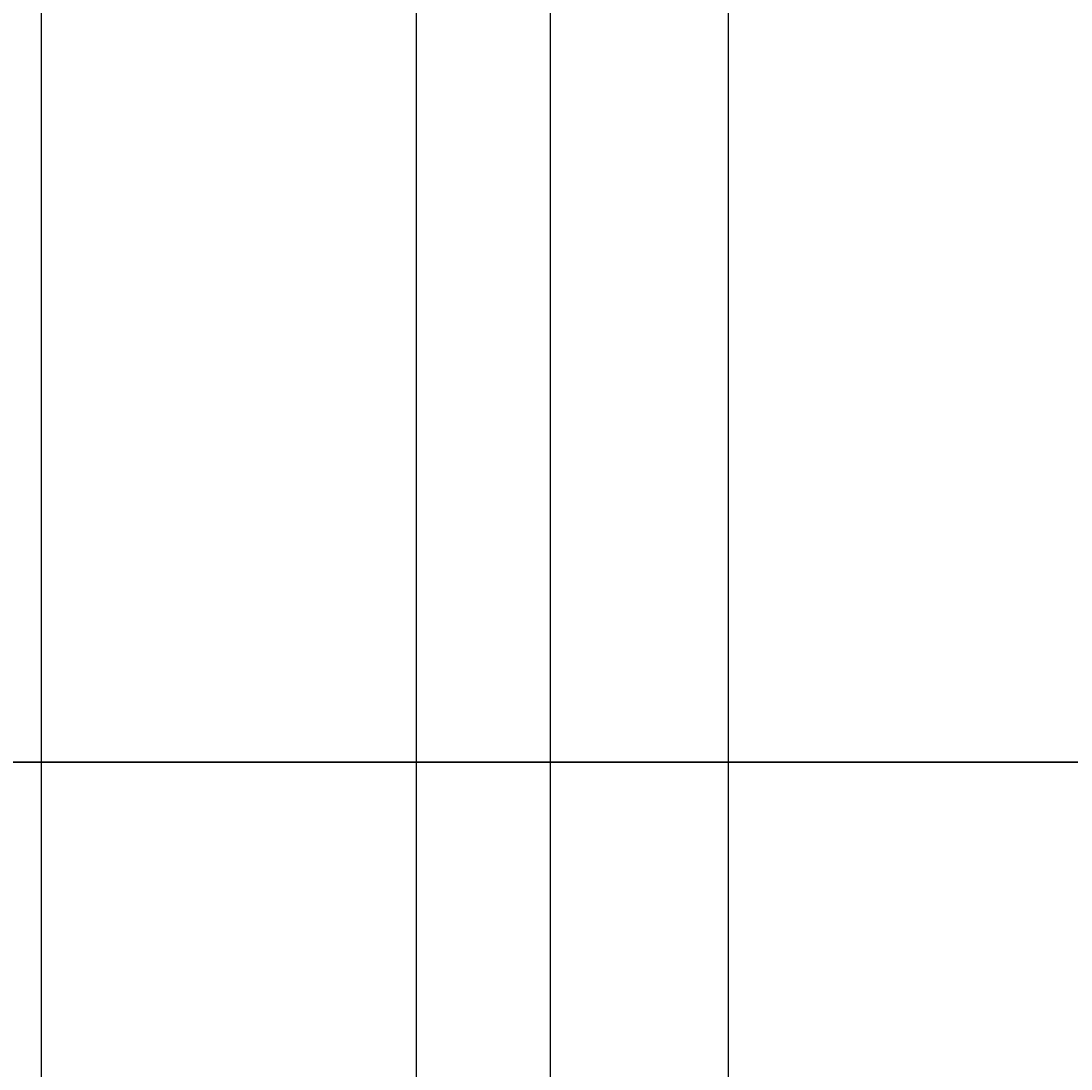
# Model space of a CAD drawing. Units: inches. Extents: x -6 to 289, y -8 to 323.
# Tile 80 of 107: x 126 to 150, y 252 to 276. Entities that reach past the tile are written whole.
import ezdxf

# ---------------------------------------------------------------- set-up
doc = ezdxf.new("R2010")
doc.units = ezdxf.units.IN
doc.header["$MEASUREMENT"] = 0
doc.layers.add('A-ANNO-DIMS', color=2, linetype='Continuous', lineweight=18)
doc.layers.add('A-ELEV', color=7, linetype='Continuous', lineweight=35)
doc.styles.get("Standard").update_dxf_attribs({"font": 'arial.ttf'})
doc.dimstyles.get("Standard").update_dxf_attribs({"dimtxt": 0.18, "dimasz": 0.18, "dimexe": 0.18, "dimexo": 0.0625, "dimgap": 0.09, "dimtad": 0, "dimtih": 1, "dimtoh": 1, "dimdec": 4, "dimzin": 0, "dimdsep": 46, "dimtxsty": 'Standard', "dimcen": 0.09, "dimadec": 0, "dimazin": 0, "dimtfac": 1, "dimtdec": 4, "dimtofl": 0, "dimtmove": 0, "dimatfit": 3, "dimfxl": 1, "dimtolj": 1, "dimtzin": 0, "dimarcsym": 0})

# ---------------------------------------------------------------- blocks, each defined once
blk = doc.blocks.new('*D10')
at = {"layer": 'A-ANNO-DIMS', "color": 0, "lineweight": -2, "transparency": 16777216}
for p, q in [((115.164, 307.351), (115.164, 322.969)), ((126.883, 226.717), (126.883, 322.969)), ((115.344, 322.789), (120.639, 322.789)), ((126.703, 322.789), (121.408, 322.789))]:
    blk.add_line(p, q, dxfattribs=at)
at = {"layer": 'A-ANNO-DIMS', "color": 0, "transparency": 16777216}
for points in [[(115.344, 322.819), (115.344, 322.759), (115.164, 322.789)], [(126.703, 322.819), (126.703, 322.759), (126.883, 322.789)]]:
    blk.add_solid(points, dxfattribs=at)
at = {"layer": 'Defpoints', "color": 0, "transparency": 16777216}
for p in [(126.883, 322.789), (115.164, 307.289), (126.883, 226.654)]:
    blk.add_point(p, dxfattribs=at)
at = {"layer": 'A-ANNO-DIMS', "color": 0, "transparency": 16777216, "insert": (121.024, 322.789), "char_height": 0.18, "attachment_point": 5}
blk.add_mtext('\\A1;11.72', dxfattribs=at)
blk = doc.blocks.new('*D11')
at = {"layer": 'A-ANNO-DIMS', "color": 0, "lineweight": -2, "transparency": 16777216}
for p, q in [((126.883, 226.717), (126.883, 322.969)), ((168.883, 226.717), (168.883, 322.969)), ((127.063, 322.789), (147.662, 322.789)), ((168.703, 322.789), (148.105, 322.789))]:
    blk.add_line(p, q, dxfattribs=at)
at = {"layer": 'A-ANNO-DIMS', "color": 0, "transparency": 16777216}
for points in [[(127.063, 322.819), (127.063, 322.759), (126.883, 322.789)], [(168.703, 322.819), (168.703, 322.759), (168.883, 322.789)]]:
    blk.add_solid(points, dxfattribs=at)
at = {"layer": 'Defpoints', "color": 0, "transparency": 16777216}
for p in [(168.883, 322.789), (126.883, 226.654), (168.883, 226.654)]:
    blk.add_point(p, dxfattribs=at)
at = {"layer": 'A-ANNO-DIMS', "color": 0, "transparency": 16777216, "insert": (147.883, 322.789), "char_height": 0.18, "attachment_point": 5}
blk.add_mtext('\\A1;42', dxfattribs=at)
blk = doc.blocks.new('*D27')
at = {"layer": 'A-ANNO-DIMS', "color": 0, "lineweight": -2, "transparency": 16777216}
for p, q in [((19.226, 307.289), (288.653, 307.289)), ((288.473, 307.109), (288.473, 277.471)), ((288.473, 247.469), (288.473, 277.107)), ((247.226, 247.289), (288.653, 247.289))]:
    blk.add_line(p, q, dxfattribs=at)
at = {"layer": 'A-ANNO-DIMS', "color": 0, "transparency": 16777216}
for points in [[(288.443, 307.109), (288.503, 307.109), (288.473, 307.289)], [(288.443, 247.469), (288.503, 247.469), (288.473, 247.289)]]:
    blk.add_solid(points, dxfattribs=at)
at = {"layer": 'Defpoints', "color": 0, "transparency": 16777216}
for p in [(19.164, 307.289), (288.473, 307.289), (247.164, 247.289)]:
    blk.add_point(p, dxfattribs=at)
at = {"layer": 'A-ANNO-DIMS', "color": 0, "transparency": 16777216, "insert": (288.473, 277.289), "char_height": 0.18, "attachment_point": 5}
blk.add_mtext('\\A1;60', dxfattribs=at)
blk = doc.blocks.new('*D73')
at = {"layer": 'A-ANNO-DIMS', "color": 0, "lineweight": -2, "transparency": 16777216}
for p, q in [((121.008, 51.148), (121.008, 322.969)), ((135.296, 51.148), (135.296, 322.969)), ((121.188, 322.789), (127.697, 322.789)), ((135.116, 322.789), (128.607, 322.789))]:
    blk.add_line(p, q, dxfattribs=at)
at = {"layer": 'A-ANNO-DIMS', "color": 0, "transparency": 16777216}
for points in [[(121.188, 322.819), (121.188, 322.759), (121.008, 322.789)], [(135.116, 322.819), (135.116, 322.759), (135.296, 322.789)]]:
    blk.add_solid(points, dxfattribs=at)
at = {"layer": 'Defpoints', "color": 0, "transparency": 16777216}
for p in [(135.296, 322.789), (121.008, 51.085), (135.296, 51.085)]:
    blk.add_point(p, dxfattribs=at)
at = {"layer": 'A-ANNO-DIMS', "color": 0, "transparency": 16777216, "insert": (128.152, 322.789), "char_height": 0.18, "attachment_point": 5}
blk.add_mtext('\\A1;14.288', dxfattribs=at)
blk = doc.blocks.new('*D74')
at = {"layer": 'A-ANNO-DIMS', "color": 0, "lineweight": -2, "transparency": 16777216}
for p, q in [((135.296, 51.148), (135.296, 322.969)), ((138.296, 51.148), (138.296, 322.969)), ((135.476, 322.789), (136.647, 322.789)), ((138.116, 322.789), (136.945, 322.789))]:
    blk.add_line(p, q, dxfattribs=at)
at = {"layer": 'A-ANNO-DIMS', "color": 0, "transparency": 16777216}
for points in [[(135.476, 322.819), (135.476, 322.759), (135.296, 322.789)], [(138.116, 322.819), (138.116, 322.759), (138.296, 322.789)]]:
    blk.add_solid(points, dxfattribs=at)
at = {"layer": 'Defpoints', "color": 0, "transparency": 16777216}
for p in [(138.296, 322.789), (135.296, 51.085), (138.296, 51.085)]:
    blk.add_point(p, dxfattribs=at)
at = {"layer": 'A-ANNO-DIMS', "color": 0, "transparency": 16777216, "insert": (136.796, 322.789), "char_height": 0.18, "attachment_point": 5}
blk.add_mtext('\\A1;3', dxfattribs=at)
blk = doc.blocks.new('*D75')
at = {"layer": 'A-ANNO-DIMS', "color": 0, "lineweight": -2, "transparency": 16777216}
for p, q in [((138.296, 51.148), (138.296, 322.969)), ((142.296, 51.148), (142.296, 322.969)), ((138.476, 322.789), (140.144, 322.789)), ((142.116, 322.789), (140.448, 322.789))]:
    blk.add_line(p, q, dxfattribs=at)
at = {"layer": 'A-ANNO-DIMS', "color": 0, "transparency": 16777216}
for points in [[(138.476, 322.819), (138.476, 322.759), (138.296, 322.789)], [(142.116, 322.819), (142.116, 322.759), (142.296, 322.789)]]:
    blk.add_solid(points, dxfattribs=at)
at = {"layer": 'Defpoints', "color": 0, "transparency": 16777216}
for p in [(142.296, 322.789), (138.296, 51.085), (142.296, 51.085)]:
    blk.add_point(p, dxfattribs=at)
at = {"layer": 'A-ANNO-DIMS', "color": 0, "transparency": 16777216, "insert": (140.296, 322.789), "char_height": 0.18, "attachment_point": 5}
blk.add_mtext('\\A1;4', dxfattribs=at)
blk = doc.blocks.new('*D76')
at = {"layer": 'A-ANNO-DIMS', "color": 0, "lineweight": -2, "transparency": 16777216}
for p, q in [((142.296, 51.148), (142.296, 322.969)), ((164.296, 51.148), (164.296, 322.969)), ((142.476, 322.789), (153.076, 322.789)), ((164.116, 322.789), (153.516, 322.789))]:
    blk.add_line(p, q, dxfattribs=at)
at = {"layer": 'A-ANNO-DIMS', "color": 0, "transparency": 16777216}
for points in [[(142.476, 322.819), (142.476, 322.759), (142.296, 322.789)], [(164.116, 322.819), (164.116, 322.759), (164.296, 322.789)]]:
    blk.add_solid(points, dxfattribs=at)
at = {"layer": 'Defpoints', "color": 0, "transparency": 16777216}
for p in [(164.296, 322.789), (142.296, 51.085), (164.296, 51.085)]:
    blk.add_point(p, dxfattribs=at)
at = {"layer": 'A-ANNO-DIMS', "color": 0, "transparency": 16777216, "insert": (153.296, 322.789), "char_height": 0.18, "attachment_point": 5}
blk.add_mtext('\\A1;22', dxfattribs=at)
blk = doc.blocks.new('*D94')
at = {"layer": 'A-ANNO-DIMS', "color": 0, "lineweight": -2, "transparency": 16777216}
for p, q in [((118.164, 159.411), (118.164, 322.969)), ((161.552, 159.411), (161.552, 322.969)), ((118.344, 322.789), (139.46, 322.789)), ((161.372, 322.789), (140.256, 322.789))]:
    blk.add_line(p, q, dxfattribs=at)
at = {"layer": 'A-ANNO-DIMS', "color": 0, "transparency": 16777216}
for points in [[(118.344, 322.819), (118.344, 322.759), (118.164, 322.789)], [(161.372, 322.819), (161.372, 322.759), (161.552, 322.789)]]:
    blk.add_solid(points, dxfattribs=at)
at = {"layer": 'Defpoints', "color": 0, "transparency": 16777216}
for p in [(161.552, 322.789), (118.164, 159.348), (161.552, 159.348)]:
    blk.add_point(p, dxfattribs=at)
at = {"layer": 'A-ANNO-DIMS', "color": 0, "transparency": 16777216, "insert": (139.858, 322.789), "char_height": 0.18, "attachment_point": 5}
blk.add_mtext('\\A1;43.39', dxfattribs=at)

msp = doc.modelspace()

# ---------------------------------------------------------------- linework, layer by layer
at = {"layer": 'A-ELEV'}
msp.add_line((115.1638, 259.2888), (271.1638, 259.2888), dxfattribs=at)

# ---------------------------------------------------------------- dimensions: what is measured, and where the dimension line sits
at = {"layer": 'A-ANNO-DIMS'}
for base, p1, p2, override, picture, middle in [((126.8835, 322.7888), (115.1638, 307.2888), (126.8835, 226.654), {"dimdec": 2, "dimlfac": 1, "dimrnd": 0, "dimzin": 0, "dimdsep": 46, "dimlunit": 2}, '*D10', (121.0236, 322.7888)), ((161.5522, 322.7888), (118.1638, 159.3484), (161.5522, 159.3484), {"dimdec": 2, "dimlfac": 1, "dimrnd": 0, "dimzin": 0, "dimdsep": 46, "dimlunit": 2}, '*D94', (139.858, 322.7888)), ((135.296, 322.7888), (121.008, 51.0851), (135.296, 51.0851), {"dimdec": 3, "dimlfac": 1, "dimrnd": 0, "dimzin": 0, "dimdsep": 46, "dimlunit": 2}, '*D73', (128.152, 322.7888)), ((168.8835, 322.7888), (126.8835, 226.654), (168.8835, 226.654), {"dimdec": 0, "dimlfac": 1, "dimrnd": 0, "dimzin": 0, "dimdsep": 46, "dimlunit": 2}, '*D11', (147.8835, 322.7888)), ((138.296, 322.7888), (135.296, 51.0851), (138.296, 51.0851), {"dimdec": 0, "dimlfac": 1, "dimrnd": 0, "dimzin": 0, "dimdsep": 46, "dimlunit": 2}, '*D74', (136.796, 322.7888)), ((142.296, 322.7888), (138.296, 51.0851), (142.296, 51.0851), {"dimdec": 0, "dimlfac": 1, "dimrnd": 0, "dimzin": 0, "dimdsep": 46, "dimlunit": 2}, '*D75', (140.296, 322.7888)), ((164.296, 322.7888), (142.296, 51.0851), (164.296, 51.0851), {"dimdec": 0, "dimlfac": 1, "dimrnd": 0, "dimzin": 0, "dimdsep": 46, "dimlunit": 2}, '*D76', (153.296, 322.7888))]:
    dim = msp.add_linear_dim(base=base, p1=p1, p2=p2, dimstyle='Standard', override=override, dxfattribs=at)
    dim.commit()
    dim.dimension.update_dxf_attribs({"geometry": picture, "text_midpoint": middle})
dim = msp.add_linear_dim(base=(288.4733, 307.2888), p1=(247.1638, 247.2888), p2=(19.1638, 307.2888), angle=90, dimstyle='Standard', override={"dimdec": 0, "dimlfac": 1, "dimrnd": 0, "dimzin": 0, "dimdsep": 46, "dimlunit": 2}, dxfattribs=at)
dim.commit()
dim.dimension.update_dxf_attribs({"geometry": '*D27', "text_midpoint": (288.4733, 277.2888)})

doc.saveas('drawing.dxf')
